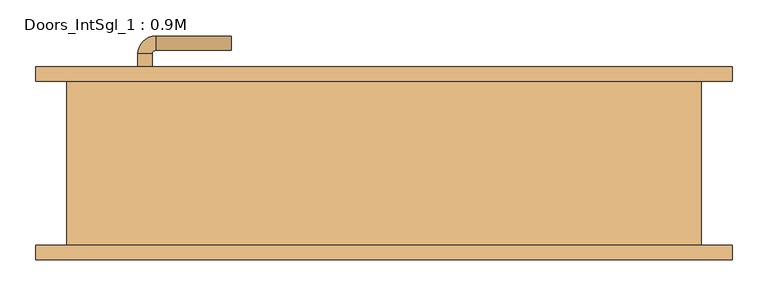
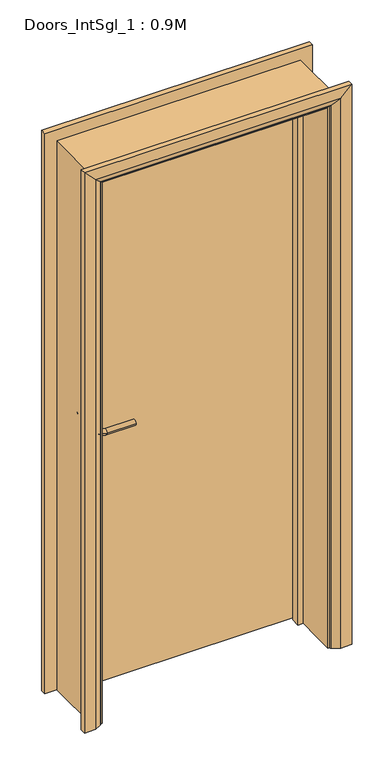
"""IFC4 building model written with IfcOpenShell, lengths in millimetres: door geometry, Doors_IntSgl_1 : 0.9M."""

from ifc_helpers import new_model, si_unit, point, frame, frame_2d, origin, place, context, project, spatial, polyline, circle_curve, ellipse_curve, trimmed, segment, composite_curve, outline, extrude, faceted_brep, source, transform, mapped, element, save
from ifc_brep_helpers import plane_surface, cylinder_surface, revolved_surface, advanced_brep


def doors_intsgl_1_0_9m_a04e9bb1(model_context):
    return source(origin(), model_context, "Body", "SolidModel", [
        advanced_brep(
        [(-343.0, 68.3, 1000.0), (-323.0, 68.3, 1000.0), (-323.0, 38.3, 1000.0), (-343.0, 38.3, 1000.0), (-318.0, 33.3, 1000.0), (-318.0, 13.3, 1000.0), (-213.0, 13.3, 1000.0), (-213.0, 33.3, 1000.0)],
        [
            (0, 1, circle_curve(frame((-333.0, 68.3, 1000.0), z_axis=(0.0, 1.0, 0.0), x_axis=(1.0, 0.0, 0.0)), 10.0)),
            (1, 0, circle_curve(frame((-333.0, 68.3, 1000.0), z_axis=(0.0, 1.0, 0.0), x_axis=(1.0, 0.0, 0.0)), 10.0)),
            (1, 2),
            (2, 3, circle_curve(frame((-333.0, 38.3, 1000.0), z_axis=(0.0, 1.0, 0.0), x_axis=(1.0, 0.0, 0.0)), 10.0)),
            (3, 0),
            (3, 2, circle_curve(frame((-333.0, 38.3, 1000.0), z_axis=(0.0, 1.0, 0.0), x_axis=(1.0, 0.0, 0.0)), 10.0)),
            (4, 5, circle_curve(frame((-318.0, 23.3, 1000.0), z_axis=(-1.0, 0.0, 0.0), x_axis=(0.0, 1.0, 0.0)), 10.0)),
            (5, 3, circle_curve(frame((-318.0, 38.3, 1000.0), z_axis=(0.0, 0.0, -1.0), x_axis=(-1.0, 0.0, 0.0)), 25.0)),
            (2, 4, circle_curve(frame((-318.0, 38.3, 1000.0), z_axis=(0.0, 0.0, 1.0), x_axis=(-1.0, 0.0, 0.0)), 5.0)),
            (5, 4, circle_curve(frame((-318.0, 23.3, 1000.0), z_axis=(-1.0, 0.0, 0.0), x_axis=(0.0, 1.0, 0.0)), 10.0)),
            (6, 7, circle_curve(frame((-213.0, 23.3, 1000.0), z_axis=(1.0, 0.0, 0.0), x_axis=(0.0, 1.0, 0.0)), 10.0)),
            (7, 6, circle_curve(frame((-213.0, 23.3, 1000.0), z_axis=(1.0, 0.0, 0.0), x_axis=(0.0, 1.0, 0.0)), 10.0)),
            (4, 7),
            (6, 5),
        ],
        [
            plane_surface(frame((-333.0, 68.3, 1000.0), z_axis=(0.0, 1.0, 0.0), x_axis=(0.0, 0.0, 1.0))),
            cylinder_surface(frame((-333.0, 68.3, 1000.0), z_axis=(0.0, 1.0, 0.0), x_axis=(1.0, 0.0, 0.0)), 10.0),
            revolved_surface(trimmed(ellipse_curve(frame((-333.0, 38.3, 1000.0), z_axis=(0.0, -1.0, 0.0), x_axis=(1.0, 0.0, 0.0)), 10.0, 10.0), [point((-343.0, 38.3, 1000.0))], [point((-323.0, 38.3, 1000.0))], True, "CARTESIAN"), (-318.0, 38.3, 1000.0), (0.0, 0.0, -1.0)),
            revolved_surface(trimmed(ellipse_curve(frame((-333.0, 38.3, 1000.0), z_axis=(0.0, -1.0, 0.0), x_axis=(1.0, 0.0, 0.0)), 10.0, 10.0), [point((-323.0, 38.3, 1000.0))], [point((-343.0, 38.3, 1000.0))], True, "CARTESIAN"), (-318.0, 38.3, 1000.0), (0.0, 0.0, -1.0)),
            plane_surface(frame((-213.0, 23.3, 1000.0), z_axis=(1.0, 0.0, 0.0), x_axis=(0.0, 0.0, 1.0))),
            cylinder_surface(frame((-318.0, 23.3, 1000.0), z_axis=(-1.0, 0.0, 0.0), x_axis=(0.0, 1.0, 0.0)), 10.0),
        ],
        [
            (0, [[1, 2]]),
            (1, [[3, 4, 5, -2]]),
            (1, [[-5, 6, -3, -1]]),
            (2, [[7, 8, -4, 9]]),
            (3, [[10, -9, -6, -8]]),
            (4, [[11, 12]]),
            (5, [[13, -11, 14, -7]]),
            (5, [[-14, -12, -13, -10]]),
        ],
    ),
        extrude(outline(composite_curve([segment(trimmed(circle_curve(frame_2d((1000.0, -335.5)), 30.0), [point((1000.0, -365.5))], [point((1000.0, -305.5))], False, "CARTESIAN"), True, "CONTINUOUS"), segment(trimmed(circle_curve(frame_2d((1000.0, -335.5)), 30.0), [point((1000.0, -305.5))], [point((1000.0, -365.5))], False, "CARTESIAN"), True, "CONTINUOUS")], self_intersect=False)), frame((0.0, 68.3, 0.0), z_axis=(0.0, 1.0, 0.0), x_axis=(0.0, 0.0, 1.0)), (0.0, 0.0, 1.0), 8.0),
        advanced_brep(
        [(-343.0, 122.3, 1000.0), (-323.0, 122.3, 1000.0), (-343.0, 152.3, 1000.0), (-323.0, 152.3, 1000.0), (-318.0, 157.3, 1000.0), (-318.0, 177.3, 1000.0), (-213.0, 177.3, 1000.0), (-213.0, 157.3, 1000.0)],
        [
            (0, 1, circle_curve(frame((-333.0, 122.3, 1000.0), z_axis=(0.0, -1.0, 0.0), x_axis=(1.0, 0.0, 0.0)), 10.0)),
            (1, 0, circle_curve(frame((-333.0, 122.3, 1000.0), z_axis=(0.0, -1.0, 0.0), x_axis=(1.0, 0.0, 0.0)), 10.0)),
            (0, 2),
            (2, 3, circle_curve(frame((-333.0, 152.3, 1000.0), z_axis=(0.0, -1.0, 0.0), x_axis=(1.0, 0.0, 0.0)), 10.0)),
            (3, 1),
            (3, 2, circle_curve(frame((-333.0, 152.3, 1000.0), z_axis=(0.0, -1.0, 0.0), x_axis=(1.0, 0.0, 0.0)), 10.0)),
            (4, 3, circle_curve(frame((-318.0, 152.3, 1000.0), z_axis=(0.0, 0.0, 1.0), x_axis=(-1.0, 0.0, 0.0)), 5.0)),
            (2, 5, circle_curve(frame((-318.0, 152.3, 1000.0), z_axis=(0.0, 0.0, -1.0), x_axis=(-1.0, 0.0, 0.0)), 25.0)),
            (5, 4, circle_curve(frame((-318.0, 167.3, 1000.0), z_axis=(-1.0, 0.0, 0.0), x_axis=(0.0, -1.0, 0.0)), 10.0)),
            (4, 5, circle_curve(frame((-318.0, 167.3, 1000.0), z_axis=(-1.0, 0.0, 0.0), x_axis=(0.0, -1.0, 0.0)), 10.0)),
            (6, 7, circle_curve(frame((-213.0, 167.3, 1000.0), z_axis=(1.0, 0.0, 0.0), x_axis=(0.0, -1.0, 0.0)), 10.0)),
            (7, 6, circle_curve(frame((-213.0, 167.3, 1000.0), z_axis=(1.0, 0.0, 0.0), x_axis=(0.0, -1.0, 0.0)), 10.0)),
            (5, 6),
            (7, 4),
        ],
        [
            plane_surface(frame((-333.0, 122.3, 1000.0), z_axis=(0.0, -1.0, 0.0), x_axis=(0.0, 0.0, 1.0))),
            cylinder_surface(frame((-333.0, 122.3, 1000.0), z_axis=(0.0, -1.0, 0.0), x_axis=(1.0, 0.0, 0.0)), 10.0),
            revolved_surface(trimmed(ellipse_curve(frame((-333.0, 152.3, 1000.0), z_axis=(0.0, -1.0, 0.0), x_axis=(1.0, 0.0, 0.0)), 10.0, 10.0), [point((-343.0, 152.3, 1000.0))], [point((-323.0, 152.3, 1000.0))], True, "CARTESIAN"), (-318.0, 152.3, 1000.0), (0.0, 0.0, -1.0)),
            revolved_surface(trimmed(ellipse_curve(frame((-333.0, 152.3, 1000.0), z_axis=(0.0, -1.0, 0.0), x_axis=(1.0, 0.0, 0.0)), 10.0, 10.0), [point((-323.0, 152.3, 1000.0))], [point((-343.0, 152.3, 1000.0))], True, "CARTESIAN"), (-318.0, 152.3, 1000.0), (0.0, 0.0, -1.0)),
            plane_surface(frame((-213.0, 167.3, 1000.0), z_axis=(1.0, 0.0, 0.0), x_axis=(0.0, 0.0, 1.0))),
            cylinder_surface(frame((-318.0, 167.3, 1000.0), z_axis=(-1.0, 0.0, 0.0), x_axis=(0.0, -1.0, 0.0)), 10.0),
        ],
        [
            (0, [[1, 2]]),
            (1, [[-1, 3, 4, 5]]),
            (1, [[-2, -5, 6, -3]]),
            (2, [[7, -4, 8, 9]]),
            (3, [[-8, -6, -7, 10]]),
            (4, [[11, 12]]),
            (5, [[-9, 13, -12, 14]]),
            (5, [[-10, -14, -11, -13]]),
        ],
    ),
        extrude(outline(composite_curve([segment(trimmed(circle_curve(frame_2d((1000.0, -335.5)), 30.0), [point((1000.0, -365.5))], [point((1000.0, -305.5))], False, "CARTESIAN"), True, "CONTINUOUS"), segment(trimmed(circle_curve(frame_2d((1000.0, -335.5)), 30.0), [point((1000.0, -305.5))], [point((1000.0, -365.5))], False, "CARTESIAN"), True, "CONTINUOUS")], self_intersect=False)), frame((0.0, 114.3, 0.0), z_axis=(0.0, 1.0, 0.0), x_axis=(0.0, 0.0, 1.0)), (0.0, 0.0, 1.0), 8.0),
        extrude(outline(polyline([(408.0, 76.3), (-408.0, 76.3), (-408.0, 114.3), (408.0, 114.3), (408.0, 76.3)])), frame((0.0, 0.0, 8.0), z_axis=(0.0, 0.0, 1.0), x_axis=(1.0, 0.0, 0.0)), (0.0, 0.0, 1.0), 2060.0),
        faceted_brep([(-410.0, 114.3, 0.0), (-410.0, -114.3, 0.0), (-442.0, -114.3, 0.0), (-442.0, 114.3, 0.0), (-410.0, 114.3, 2070.0), (-410.0, -114.3, 2070.0), (-442.0, -114.3, 2102.0), (-442.0, 114.3, 2102.0), (410.0, 114.3, 0.0), (442.0, 114.3, 0.0), (442.0, -114.3, 0.0), (410.0, -114.3, 0.0), (410.0, 114.3, 2070.0), (442.0, 114.3, 2102.0), (442.0, -114.3, 2102.0), (410.0, -114.3, 2070.0)], [[[0, 1, 2, 3]], [[1, 0, 4, 5]], [[2, 1, 5, 6]], [[3, 2, 6, 7]], [[0, 3, 7, 4]], [[8, 9, 10, 11]], [[12, 13, 9, 8]], [[13, 14, 10, 9]], [[14, 15, 11, 10]], [[15, 12, 8, 11]], [[5, 4, 12, 15]], [[6, 5, 15, 14]], [[7, 6, 14, 13]], [[4, 7, 13, 12]]]),
        advanced_brep(
        [(-485.0, -134.3, 0.0), (-485.0, -114.3, 0.0), (-415.0, -114.3, 0.0), (-419.0, -120.3, 0.0), (-445.0, -134.3, 0.0), (-485.0, -134.3, 2145.0), (-485.0, -114.3, 2145.0), (-415.0, -114.3, 2075.0), (-419.0, -120.3, 2079.0), (-445.0, -134.3, 2105.0), (485.0, -134.3, 0.0), (445.0, -134.3, 0.0), (419.0, -120.3, 0.0), (415.0, -114.3, 0.0), (485.0, -114.3, 0.0), (485.0, -134.3, 2145.0), (445.0, -134.3, 2105.0), (419.0, -120.3, 2079.0), (415.0, -114.3, 2075.0), (485.0, -114.3, 2145.0)],
        [
            (0, 1),
            (1, 2),
            (2, 3, circle_curve(frame((-423.0, -113.3, 0.0), z_axis=(0.0, 0.0, -1.0), x_axis=(-1.0, 0.0, 0.0)), 8.0622577)),
            (3, 4),
            (4, 0),
            (0, 5),
            (5, 6),
            (6, 1),
            (6, 7),
            (7, 2),
            (7, 8, ellipse_curve(frame((-423.0, -113.3, 2083.0), z_axis=(-0.7071067811865475, 0.0, -0.7071067811865475), x_axis=(0.7071067811865474, 0.0, -0.7071067811865476)), 11.4017543, 8.0622577)),
            (8, 3),
            (8, 9),
            (9, 4),
            (9, 5),
            (10, 11),
            (11, 12),
            (12, 13, circle_curve(frame((423.0, -113.3, 0.0), z_axis=(0.0, 0.0, -1.0), x_axis=(1.0, 0.0, 0.0)), 8.0622577)),
            (13, 14),
            (14, 10),
            (15, 16),
            (16, 11),
            (10, 15),
            (16, 17),
            (17, 12),
            (17, 18, ellipse_curve(frame((423.0, -113.3, 2083.0), z_axis=(0.7071067811865475, 0.0, -0.7071067811865475), x_axis=(0.7071067811865474, 0.0, 0.7071067811865476)), 11.4017543, 8.0622577)),
            (18, 13),
            (18, 19),
            (19, 14),
            (19, 15),
            (5, 15),
            (19, 6),
            (18, 7),
            (17, 8),
            (16, 9),
        ],
        [
            plane_surface(frame((-415.0, -187.1010989, 0.0), z_axis=(0.0, 0.0, -1.0), x_axis=(1.0, 0.0, 0.0))),
            plane_surface(frame((-485.0, -134.3, 0.0), z_axis=(-1.0, 0.0, 0.0), x_axis=(0.0, 0.0, 1.0))),
            plane_surface(frame((-485.0, -114.3, 0.0), z_axis=(0.0, 1.0, 0.0), x_axis=(0.0, 0.0, 1.0))),
            cylinder_surface(frame((-423.0, -113.3, 0.0), z_axis=(0.0, 0.0, -1.0), x_axis=(-1.0, 0.0, 0.0)), 8.0622577),
            plane_surface(frame((-419.0, -120.3, 0.0), z_axis=(0.4740998230350183, -0.8804710999221749, 0.0), x_axis=(0.0, 0.0, 1.0))),
            plane_surface(frame((-445.0, -134.3, 0.0), z_axis=(0.0, -1.0, 0.0), x_axis=(0.0, 0.0, 1.0))),
            plane_surface(frame((415.0, -187.1010989, 0.0), z_axis=(0.0, 0.0, -1.0), x_axis=(-1.0, 0.0, 0.0))),
            plane_surface(frame((445.0, -134.3, 2105.0), z_axis=(0.0, -1.0, 0.0), x_axis=(0.0, 0.0, -1.0))),
            plane_surface(frame((419.0, -120.3, 2079.0), z_axis=(-0.4740998230350183, -0.8804710999221749, 0.0), x_axis=(0.0, 0.0, -1.0))),
            cylinder_surface(frame((423.0, -113.3, 2075.0), z_axis=(0.0, 0.0, 1.0), x_axis=(1.0, 0.0, 0.0)), 8.0622577),
            plane_surface(frame((485.0, -114.3, 2145.0), z_axis=(0.0, 1.0, 0.0), x_axis=(0.0, 0.0, -1.0))),
            plane_surface(frame((485.0, -134.3, 2145.0), z_axis=(1.0, 0.0, 0.0), x_axis=(0.0, 0.0, -1.0))),
            plane_surface(frame((-485.0, -134.3, 2145.0), z_axis=(0.0, 0.0, 1.0), x_axis=(1.0, 0.0, 0.0))),
            plane_surface(frame((-485.0, -114.3, 2145.0), z_axis=(0.0, 1.0, 0.0), x_axis=(1.0, 0.0, 0.0))),
            cylinder_surface(frame((-415.0, -113.3, 2083.0), z_axis=(-1.0, 0.0, 0.0), x_axis=(0.0, 0.0, 1.0)), 8.0622577),
            plane_surface(frame((-419.0, -120.3, 2079.0), z_axis=(0.0, -0.8804710999221749, -0.4740998230350183), x_axis=(1.0, 0.0, 0.0))),
            plane_surface(frame((-445.0, -134.3, 2105.0), z_axis=(0.0, -1.0, 0.0), x_axis=(1.0, 0.0, 0.0))),
        ],
        [
            (0, [[1, 2, 3, 4, 5]]),
            (1, [[-1, 6, 7, 8]]),
            (2, [[-2, -8, 9, 10]]),
            (3, [[-3, -10, 11, 12]]),
            (4, [[-4, -12, 13, 14]]),
            (5, [[-5, -14, 15, -6]]),
            (6, [[16, 17, 18, 19, 20]]),
            (7, [[21, 22, -16, 23]]),
            (8, [[24, 25, -17, -22]]),
            (9, [[26, 27, -18, -25]]),
            (10, [[28, 29, -19, -27]]),
            (11, [[30, -23, -20, -29]]),
            (12, [[-7, 31, -30, 32]]),
            (13, [[-9, -32, -28, 33]]),
            (14, [[-11, -33, -26, 34]]),
            (15, [[-13, -34, -24, 35]]),
            (16, [[-15, -35, -21, -31]]),
        ],
    ),
        extrude(outline(polyline([(0.0, -410.0), (0.0, -391.0), (2051.0, -391.0), (2051.0, 391.0), (0.0, 391.0), (0.0, 410.0), (2070.0, 410.0), (2070.0, -410.0), (0.0, -410.0)])), frame((0.0, 42.3, 0.0), z_axis=(0.0, 1.0, 0.0), x_axis=(0.0, 0.0, 1.0)), (0.0, 0.0, 1.0), 32.0),
        advanced_brep(
        [(485.0, 134.3, 0.0), (485.0, 114.3, 0.0), (415.0, 114.3, 0.0), (419.0, 120.3, 0.0), (445.0, 134.3, 0.0), (485.0, 134.3, 2145.0), (485.0, 114.3, 2145.0), (-485.0, 114.3, 2145.0), (-485.0, 114.3, 0.0), (-415.0, 114.3, 0.0), (-415.0, 114.3, 2075.0), (415.0, 114.3, 2075.0), (419.0, 120.3, 2079.0), (445.0, 134.3, 2105.0), (-445.0, 134.3, 2105.0), (-445.0, 134.3, 0.0), (-485.0, 134.3, 0.0), (-485.0, 134.3, 2145.0), (-419.0, 120.3, 0.0), (-419.0, 120.3, 2079.0)],
        [
            (0, 1),
            (1, 2),
            (2, 3, circle_curve(frame((423.0, 113.3, 0.0), z_axis=(0.0, 0.0, -1.0), x_axis=(1.0, 0.0, 0.0)), 8.0622577)),
            (3, 4),
            (4, 0),
            (0, 5),
            (5, 6),
            (6, 1),
            (6, 7),
            (7, 8),
            (8, 9),
            (9, 10),
            (10, 11),
            (11, 2),
            (11, 12, ellipse_curve(frame((423.0, 113.3, 2083.0), z_axis=(0.7071067811865475, 0.0, -0.7071067811865475), x_axis=(-0.7071067811865474, 0.0, -0.7071067811865476)), 11.4017543, 8.0622577)),
            (12, 3),
            (12, 13),
            (13, 4),
            (13, 14),
            (14, 15),
            (15, 16),
            (16, 17),
            (17, 5),
            (7, 17),
            (16, 8),
            (15, 18),
            (18, 9, circle_curve(frame((-423.0, 113.3, 0.0), z_axis=(0.0, 0.0, -1.0), x_axis=(-1.0, 0.0, 0.0)), 8.0622577)),
            (19, 10, ellipse_curve(frame((-423.0, 113.3, 2083.0), z_axis=(-0.7071067811865475, 0.0, -0.7071067811865475), x_axis=(-0.7071067811865474, 0.0, 0.7071067811865476)), 11.4017543, 8.0622577)),
            (18, 19),
            (14, 19),
            (19, 12),
        ],
        [
            plane_surface(frame((415.0, 114.3, 0.0), z_axis=(0.0, 0.0, -1.0), x_axis=(0.0, -1.0, 0.0))),
            plane_surface(frame((485.0, 134.3, 0.0), z_axis=(1.0, 0.0, 0.0), x_axis=(0.0, 0.0, 1.0))),
            plane_surface(frame((485.0, 114.3, 0.0), z_axis=(0.0, -1.0, 0.0), x_axis=(0.0, 0.0, 1.0))),
            cylinder_surface(frame((423.0, 113.3, 0.0), z_axis=(0.0, 0.0, -1.0), x_axis=(1.0, 0.0, 0.0)), 8.0622577),
            plane_surface(frame((419.0, 120.3, 0.0), z_axis=(-0.4740998230350126, 0.880471099922178, 0.0), x_axis=(0.0, 0.0, 1.0))),
            plane_surface(frame((445.0, 134.3, 0.0), z_axis=(0.0, 1.0, 0.0), x_axis=(0.0, 0.0, 1.0))),
            plane_surface(frame((-485.0, 134.3, 2145.0), z_axis=(-1.0, 0.0, 0.0), x_axis=(0.0, 0.0, -1.0))),
            plane_surface(frame((-415.0, 114.3, 0.0), z_axis=(0.0, 0.0, -1.0), x_axis=(0.0, -1.0, 0.0))),
            cylinder_surface(frame((-423.0, 113.3, 2075.0), z_axis=(0.0, 0.0, 1.0), x_axis=(-1.0, 0.0, 0.0)), 8.0622577),
            plane_surface(frame((-419.0, 120.3, 2079.0), z_axis=(0.47409982303501824, 0.8804710999221749, 0.0), x_axis=(0.0, 0.0, -1.0))),
            plane_surface(frame((485.0, 134.3, 2145.0), z_axis=(0.0, 0.0, 1.0), x_axis=(-1.0, 0.0, 0.0))),
            cylinder_surface(frame((415.0, 113.3, 2083.0), z_axis=(1.0, 0.0, 0.0), x_axis=(0.0, 0.0, 1.0)), 8.0622577),
            plane_surface(frame((419.0, 120.3, 2079.0), z_axis=(0.0, 0.8804710999221764, -0.4740998230350154), x_axis=(-1.0, 0.0, 0.0))),
        ],
        [
            (0, [[1, 2, 3, 4, 5]]),
            (1, [[-1, 6, 7, 8]]),
            (2, [[-2, -8, 9, 10, 11, 12, 13, 14]]),
            (3, [[-3, -14, 15, 16]]),
            (4, [[-4, -16, 17, 18]]),
            (5, [[-5, -18, 19, 20, 21, 22, 23, -6]]),
            (6, [[24, -22, 25, -10]]),
            (7, [[-21, 26, 27, -11, -25]]),
            (8, [[28, -12, -27, 29]]),
            (9, [[30, -29, -26, -20]]),
            (10, [[-7, -23, -24, -9]]),
            (11, [[-15, -13, -28, 31]]),
            (12, [[-17, -31, -30, -19]]),
        ],
    ),
    ])


if __name__ == "__main__":
    model = new_model("IFC4")
    model_context = context("Model", 3, world=origin())
    ifc_project = project(units=[si_unit("LENGTHUNIT", "METRE", prefix="MILLI")], contexts=[model_context])
    site = spatial("IfcSite", under=ifc_project)
    building = spatial("IfcBuilding", under=site)
    placement = place(None, origin())
    doors_intsgl_1_0_9m_shape = doors_intsgl_1_0_9m_a04e9bb1(model_context)
    element("IfcDoor", 1, ObjectType="Doors_IntSgl_1 : 0.9M", at=placement, inside=building, context=model_context, shape_type="MappedRepresentation", body=[
        mapped(doors_intsgl_1_0_9m_shape, transform((0.0, 0.0, 0.0), x_axis=(1.0, 0.0, 0.0), y_axis=(0.0, 1.0, 0.0), z_axis=(0.0, 0.0, 1.0))),
    ])
    save(model, "model.ifc")

# Revit data of these elements
# Type "Doors_IntSgl_1 : 0.9M"
#   Type Mark = "57"
#   Type Comments = "Internal Single"
#   Operation = "SingleSwingRight"
#   Construction Type Id = "MDOOR"
#   Manufacturer = "Revit"
#   Keynote = "L20"
#   Description = "Internal Single Door"
#   Analytic Construction = "Metal"
#   UnderCut = 0.008 m
#   Tolerance = 0.002 m
#   Thickness = 0.038 m
#   Structural Tolerance = 0.008 m
#   StopDepth = 0.032 m
#   Stop Thickness = 0.019 m
#   Rough Width = 0.9 m
#   Rough Height = 2.11 m
#   Height to Top Lock Rail = 1.0 m
#   Heat Transfer Coefficient (U) = 3.7021 W/(m²·K)
#   Handle Z Distance = 1.0 m
#   Handle X Distance = 0.075 m
#   Frame Thickness = 0.032 m
#   Door Panel Width = 0.816 m
#   Door Panel Thickness = 0.038 m
#   Door Panel Offset = 0.0 m
#   Height = 2.11 m
#   Width = 0.9 m
#   Door Panel Height = 2.06 m
#   Architrave Setback = 0.005 m
#   Vis - Ironmongery = yes
#   Define Thermal Properties by = 1
#   Material Ironmongery = Door - Handle
#   Material Frame = Door - Frame/Mullion
#   Material Door = Door - Panel
#   Material Architrave = Door - Architrave
#   Visual Light Transmittance = 0
#   Solar Heat Gain Coefficient = 0
#   Function = (empty or 0)
#   Wall Closure = (empty or 0)
# Element 1 (IfcDoor, "Doors_IntSgl_1 : 0.9M")
#   Materials on its faces: "Door - Architrave", "Door - Handle", "Door - Frame/Mullion", "Door - Panel"
# Materials
#   "Door - Handle": colour RGB 0 0 0, transparency 0, Keynote = "P21", Cost = 0
#   "Door - Frame/Mullion": class "Wood", colour RGB 212 179 113, transparency 0, Keynote = "L20", Cost = 0
#   "Door - Panel": class "Wood", colour RGB 210 159 95, transparency 0, Keynote = "L20", Cost = 0
#   "Door - Architrave": class "Wood", colour RGB 154 90 5, transparency 0, Keynote = "P20", Cost = 0
